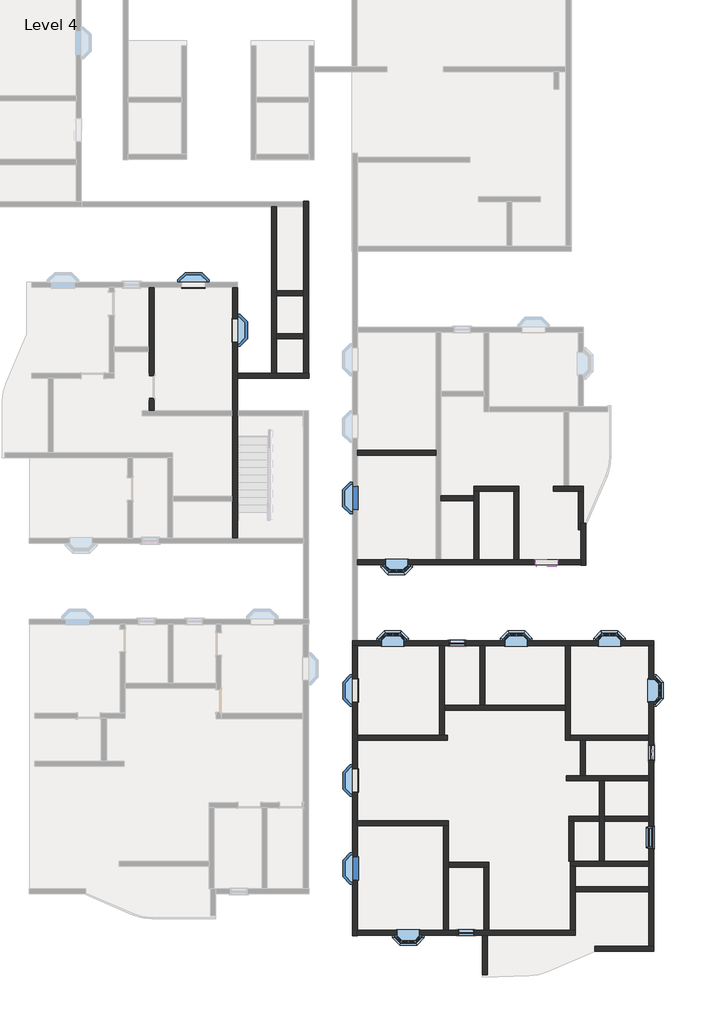
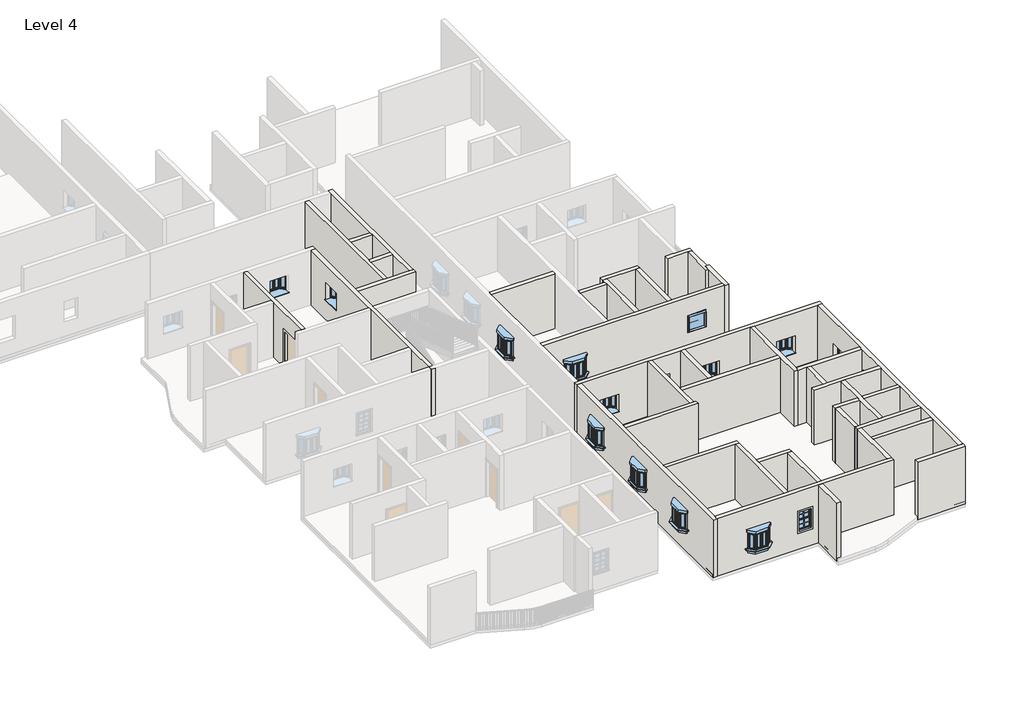
# One storey, part 2 of 14: 40 walls, 17 windows.
"""IFC4 building model written with IfcOpenShell, lengths in millimetres."""

from ifc_helpers import new_model, si_unit, frame, origin, place, context, project, spatial, polyline, outline, extrude, faceted_brep, transform, mapped, element, save
from components import window_910x910mm_67ef725a, window_8debb0fa, windows_sgl_w_glazing_bars_910x910mm_256712d0

model = new_model("IFC4")

# Units and contexts
model_context = context("Model", 3, world=origin())
ifc_project = project(units=[si_unit("LENGTHUNIT", "METRE", prefix="MILLI")], contexts=[model_context])

# Site, building, storey
site = spatial("IfcSite", under=ifc_project)
building = spatial("IfcBuilding", under=site)
storey = spatial("IfcBuildingStorey", under=building, Name="Level 4", Elevation=9144.0)

# Walls
placement = place(None, origin())
element("IfcWall", 1, ObjectType="4.5\" p", at=placement, inside=storey, context=model_context, shape_type="SweptSolid", body=[
    extrude(outline(polyline([(6070.4380523, -28382.7374148), (6070.4380523, -26796.6042694), (6273.6380523, -26796.6042694), (6273.6380523, -28382.7374148), (6070.4380523, -28382.7374148)])), frame((0.0, 0.0, 9144.0), z_axis=(0.0, 0.0, 1.0), x_axis=(1.0, 0.0, 0.0)), (0.0, 0.0, 1.0), 3048.0),
])
element("IfcWall", 2, ObjectType="4.5\" p", at=placement, inside=storey, context=model_context, shape_type="Brep", body=[
    faceted_brep([(10639.6896214, -27431.6042694, 9144.0), (13030.0380523, -27431.6042694, 9144.0), (13030.0380523, -27431.6042694, 12192.0), (10639.6896214, -27431.6042694, 12192.0), (10639.6896214, -27228.4042694, 9144.0), (10639.6896214, -27228.4042694, 12192.0), (12814.1380523, -27228.4042694, 12192.0), (13017.3380523, -27228.4042694, 12192.0), (13030.0380523, -27228.4042694, 12192.0), (13030.0380523, -27228.4042694, 9144.0), (13017.3380523, -27228.4042694, 9144.0), (12814.1380523, -27228.4042694, 9144.0)], [[[0, 1, 2, 3]], [[4, 5, 6, 7, 8, 9, 10, 11]], [[1, 0, 4, 11, 10, 9]], [[2, 1, 9, 8]], [[3, 2, 8, 7, 6, 5]], [[0, 3, 5, 4]]]),
])
element("IfcWall", 3, ObjectType="4.5\" p", at=placement, inside=storey, context=model_context, shape_type="Brep", body=[
    faceted_brep([(1015.8380523, -18878.1542694, 9144.0), (4648.0380523, -18878.1542694, 9144.0), (4648.0380523, -18878.1542694, 12192.0), (1015.8380523, -18878.1542694, 12192.0), (1015.8380523, -18674.9542694, 9144.0), (1015.8380523, -18674.9542694, 12192.0), (4336.8880523, -18674.9542694, 12192.0), (4540.0880523, -18674.9542694, 12192.0), (4648.0380523, -18674.9542694, 12192.0), (4648.0380523, -18674.9542694, 9144.0), (4540.0880523, -18674.9542694, 9144.0), (4336.8880523, -18674.9542694, 9144.0)], [[[0, 1, 2, 3]], [[4, 5, 6, 7, 8, 9, 10, 11]], [[1, 0, 4, 11, 10, 9]], [[2, 1, 9, 8]], [[3, 2, 8, 7, 6, 5]], [[0, 3, 5, 4]]]),
])
element("IfcWall", 4, ObjectType="4.5\" p", at=placement, inside=storey, context=model_context, shape_type="Brep", body=[
    faceted_brep([(4336.8880523, -15049.1042694, 9144.0), (4336.8880523, -18674.9542694, 9144.0), (4336.8880523, -18674.9542694, 12192.0), (4336.8880523, -15049.1042694, 12192.0), (4540.0880523, -15049.1042694, 9144.0), (4540.0880523, -15049.1042694, 12192.0), (4540.0880523, -17455.7542694, 12192.0), (4540.0880523, -17658.9542694, 12192.0), (4540.0880523, -18674.9542694, 12192.0), (4540.0880523, -18674.9542694, 9144.0), (4540.0880523, -17658.9542694, 9144.0), (4540.0880523, -17455.7542694, 9144.0)], [[[0, 1, 2, 3]], [[4, 5, 6, 7, 8, 9, 10, 11]], [[1, 0, 4, 11, 10, 9]], [[3, 2, 8, 7, 6, 5]], [[0, 3, 5, 4]], [[2, 1, 9, 8]]]),
])
element("IfcWall", 5, ObjectType="4.5\" p", at=placement, inside=storey, context=model_context, shape_type="Brep", body=[
    faceted_brep([(4540.0880523, -17658.9542694, 9144.0), (9442.2880523, -17658.9542694, 9144.0), (9442.2880523, -17658.9542694, 12192.0), (4540.0880523, -17658.9542694, 12192.0), (4540.0880523, -17455.7542694, 9144.0), (4540.0880523, -17455.7542694, 12192.0), (5975.1880523, -17455.7542694, 12192.0), (6178.3880523, -17455.7542694, 12192.0), (9442.2880523, -17455.7542694, 12192.0), (9442.2880523, -17455.7542694, 9144.0), (6178.3880523, -17455.7542694, 9144.0), (5975.1880523, -17455.7542694, 9144.0)], [[[0, 1, 2, 3]], [[4, 5, 6, 7, 8, 9, 10, 11]], [[1, 0, 4, 11, 10, 9]], [[3, 2, 8, 7, 6, 5]], [[0, 3, 5, 4]], [[2, 1, 9, 8]]]),
])
element("IfcWall", 6, ObjectType="4.5\" p", at=placement, inside=storey, context=model_context, shape_type="SweptSolid", body=[
    extrude(outline(polyline([(5975.1880523, -17455.7542694), (5975.1880523, -15049.1042694), (6178.3880523, -15049.1042694), (6178.3880523, -17455.7542694), (5975.1880523, -17455.7542694)])), frame((0.0, 0.0, 9144.0), z_axis=(0.0, 0.0, 1.0), x_axis=(1.0, 0.0, 0.0)), (0.0, 0.0, 1.0), 3048.0),
])
element("IfcWall", 7, ObjectType="4.5\" p", at=placement, inside=storey, context=model_context, shape_type="Brep", body=[
    faceted_brep([(9442.2880523, -15049.1042694, 9144.0), (9442.2880523, -17455.7542694, 9144.0), (9442.2880523, -17658.9542694, 9144.0), (9442.2880523, -18871.8042694, 9144.0), (9442.2880523, -18871.8042694, 12192.0), (9442.2880523, -17658.9542694, 12192.0), (9442.2880523, -17455.7542694, 12192.0), (9442.2880523, -15049.1042694, 12192.0), (9645.4880523, -15049.1042694, 9144.0), (9645.4880523, -15049.1042694, 12192.0), (9645.4880523, -18668.6042694, 12192.0), (9645.4880523, -18871.8042694, 12192.0), (9645.4880523, -18871.8042694, 9144.0), (9645.4880523, -18668.6042694, 9144.0)], [[[0, 1, 2, 3, 4, 5, 6, 7]], [[8, 9, 10, 11, 12, 13]], [[3, 2, 1, 0, 8, 13, 12]], [[7, 6, 5, 4, 11, 10, 9]], [[0, 7, 9, 8]], [[4, 3, 12, 11]]]),
])
element("IfcWall", 8, ObjectType="4.5\" p", at=placement, inside=storey, context=model_context, shape_type="Brep", body=[
    faceted_brep([(1015.8380523, -22345.2542694, 9144.0), (4489.2880523, -22345.2542694, 9144.0), (4692.4880523, -22345.2542694, 9144.0), (4692.4880523, -22345.2542694, 12192.0), (4489.2880523, -22345.2542694, 12192.0), (1015.8380523, -22345.2542694, 12192.0), (1015.8380523, -22142.0542694, 9144.0), (1015.8380523, -22142.0542694, 12192.0), (4692.4880523, -22142.0542694, 12192.0), (4692.4880523, -22142.0542694, 9144.0)], [[[0, 1, 2, 3, 4, 5]], [[6, 7, 8, 9]], [[2, 1, 0, 6, 9]], [[5, 4, 3, 8, 7]], [[0, 5, 7, 6]], [[3, 2, 9, 8]]]),
])
element("IfcWall", 9, ObjectType="4.5\" p", at=placement, inside=storey, context=model_context, shape_type="Brep", body=[
    faceted_brep([(4489.2880523, -22345.2542694, 9144.0), (4489.2880523, -26580.7042694, 9144.0), (4489.2880523, -26580.7042694, 12192.0), (4489.2880523, -22345.2542694, 12192.0), (4692.4880523, -22345.2542694, 9144.0), (4692.4880523, -22345.2542694, 12192.0), (4692.4880523, -23818.4542694, 12192.0), (4692.4880523, -24021.6542694, 12192.0), (4692.4880523, -26580.7042694, 12192.0), (4692.4880523, -26580.7042694, 9144.0), (4692.4880523, -24021.6542694, 9144.0), (4692.4880523, -23818.4542694, 9144.0)], [[[0, 1, 2, 3]], [[4, 5, 6, 7, 8, 9, 10, 11]], [[1, 0, 4, 11, 10, 9]], [[3, 2, 8, 7, 6, 5]], [[0, 3, 5, 4]], [[2, 1, 9, 8]]]),
])
element("IfcWall", 10, ObjectType="4.5\" p", at=placement, inside=storey, context=model_context, shape_type="Brep", body=[
    faceted_brep([(4692.4880523, -24021.6542694, 9144.0), (6127.5880523, -24021.6542694, 9144.0), (6330.7880523, -24021.6542694, 9144.0), (6330.7880523, -24021.6542694, 12192.0), (6127.5880523, -24021.6542694, 12192.0), (4692.4880523, -24021.6542694, 12192.0), (4692.4880523, -23818.4542694, 9144.0), (4692.4880523, -23818.4542694, 12192.0), (6330.7880523, -23818.4542694, 12192.0), (6330.7880523, -23818.4542694, 9144.0)], [[[0, 1, 2, 3, 4, 5]], [[6, 7, 8, 9]], [[2, 1, 0, 6, 9]], [[5, 4, 3, 8, 7]], [[0, 5, 7, 6]], [[3, 2, 9, 8]]]),
])
element("IfcWall", 11, ObjectType="4.5\" p", at=placement, inside=storey, context=model_context, shape_type="SweptSolid", body=[
    extrude(outline(polyline([(6127.5880523, -26580.7042694), (6127.5880523, -24021.6542694), (6330.7880523, -24021.6542694), (6330.7880523, -26580.7042694), (6127.5880523, -26580.7042694)])), frame((0.0, 0.0, 9144.0), z_axis=(0.0, 0.0, 1.0), x_axis=(1.0, 0.0, 0.0)), (0.0, 0.0, 1.0), 3048.0),
])
element("IfcWall", 12, ObjectType="4.5\" p", at=placement, inside=storey, context=model_context, shape_type="Brep", body=[
    faceted_brep([(9645.4880523, -18871.8042694, 9144.0), (10051.8880523, -18871.8042694, 9144.0), (10255.0880523, -18871.8042694, 9144.0), (12814.1380523, -18871.8042694, 9144.0), (12814.1380523, -18871.8042694, 12192.0), (10255.0880523, -18871.8042694, 12192.0), (10051.8880523, -18871.8042694, 12192.0), (9645.4880523, -18871.8042694, 12192.0), (9645.4880523, -18668.6042694, 9144.0), (9645.4880523, -18668.6042694, 12192.0), (12814.1380523, -18668.6042694, 12192.0), (12814.1380523, -18668.6042694, 9144.0)], [[[0, 1, 2, 3, 4, 5, 6, 7]], [[8, 9, 10, 11]], [[3, 2, 1, 0, 8, 11]], [[7, 6, 5, 4, 10, 9]], [[0, 7, 9, 8]], [[4, 3, 11, 10]]]),
])
element("IfcWall", 13, ObjectType="4.5\" p", at=placement, inside=storey, context=model_context, shape_type="SweptSolid", body=[
    extrude(outline(polyline([(10051.8880523, -20313.2542694), (10051.8880523, -18871.8042694), (10255.0880523, -18871.8042694), (10255.0880523, -20313.2542694), (10051.8880523, -20313.2542694)])), frame((0.0, 0.0, 9144.0), z_axis=(0.0, 0.0, 1.0), x_axis=(1.0, 0.0, 0.0)), (0.0, 0.0, 1.0), 3048.0),
])
element("IfcWall", 14, ObjectType="4.5\" p", at=placement, inside=storey, context=model_context, shape_type="Brep", body=[
    faceted_brep([(12814.1380523, -20313.2542694, 9144.0), (10255.0880523, -20313.2542694, 9144.0), (10051.8880523, -20313.2542694, 9144.0), (9486.7380523, -20313.2542694, 9144.0), (9486.7380523, -20313.2542694, 12192.0), (10051.8880523, -20313.2542694, 12192.0), (10255.0880523, -20313.2542694, 12192.0), (12814.1380523, -20313.2542694, 12192.0), (12814.1380523, -20516.4542694, 9144.0), (12814.1380523, -20516.4542694, 12192.0), (11017.0880523, -20516.4542694, 12192.0), (10813.8880523, -20516.4542694, 12192.0), (9486.7380523, -20516.4542694, 12192.0), (9486.7380523, -20516.4542694, 9144.0), (10813.8880523, -20516.4542694, 9144.0), (11017.0880523, -20516.4542694, 9144.0)], [[[0, 1, 2, 3, 4, 5, 6, 7]], [[8, 9, 10, 11, 12, 13, 14, 15]], [[3, 2, 1, 0, 8, 15, 14, 13]], [[4, 3, 13, 12]], [[7, 6, 5, 4, 12, 11, 10, 9]], [[0, 7, 9, 8]]]),
])
element("IfcWall", 15, ObjectType="4.5\" p", at=placement, inside=storey, context=model_context, shape_type="Brep", body=[
    faceted_brep([(10813.8880523, -20516.4542694, 9144.0), (10813.8880523, -21951.5542694, 9144.0), (10813.8880523, -22154.7542694, 9144.0), (10813.8880523, -23779.5416506, 9144.0), (10813.8880523, -23779.5416506, 12192.0), (10813.8880523, -22154.7542694, 12192.0), (10813.8880523, -21951.5542694, 12192.0), (10813.8880523, -20516.4542694, 12192.0), (11017.0880523, -20516.4542694, 9144.0), (11017.0880523, -20516.4542694, 12192.0), (11017.0880523, -21951.5542694, 12192.0), (11017.0880523, -22154.7542694, 12192.0), (11017.0880523, -23779.5416506, 12192.0), (11017.0880523, -23779.5416506, 9144.0), (11017.0880523, -22154.7542694, 9144.0), (11017.0880523, -21951.5542694, 9144.0)], [[[0, 1, 2, 3, 4, 5, 6, 7]], [[8, 9, 10, 11, 12, 13, 14, 15]], [[3, 2, 1, 0, 8, 15, 14, 13]], [[7, 6, 5, 4, 12, 11, 10, 9]], [[0, 7, 9, 8]], [[4, 3, 13, 12]]]),
])
element("IfcWall", 16, ObjectType="4.5\" p", at=placement, inside=storey, context=model_context, shape_type="Brep", body=[
    faceted_brep([(12814.1380523, -23779.5416506, 9144.0), (11017.0880523, -23779.5416506, 9144.0), (10813.8880523, -23779.5416506, 9144.0), (9791.5380523, -23779.5416506, 9144.0), (9632.7880523, -23779.5416506, 9144.0), (9632.7880523, -23779.5416506, 12192.0), (9791.5380523, -23779.5416506, 12192.0), (10813.8880523, -23779.5416506, 12192.0), (11017.0880523, -23779.5416506, 12192.0), (12814.1380523, -23779.5416506, 12192.0), (12814.1380523, -23982.7416506, 9144.0), (12814.1380523, -23982.7416506, 12192.0), (9835.9880523, -23982.7416506, 12192.0), (9632.7880523, -23982.7416506, 12192.0), (9632.7880523, -23982.7416506, 9144.0), (9835.9880523, -23982.7416506, 9144.0)], [[[0, 1, 2, 3, 4, 5, 6, 7, 8, 9]], [[10, 11, 12, 13, 14, 15]], [[4, 3, 2, 1, 0, 10, 15, 14]], [[9, 8, 7, 6, 5, 13, 12, 11]], [[0, 9, 11, 10]], [[5, 4, 14, 13]]]),
])
element("IfcWall", 17, ObjectType="4.5\" p", at=placement, inside=storey, context=model_context, shape_type="Brep", body=[
    faceted_brep([(9632.7880523, -23982.7416506, 9144.0), (9632.7880523, -26580.7042694, 9144.0), (9632.7880523, -26580.7042694, 12192.0), (9632.7880523, -23982.7416506, 12192.0), (9835.9880523, -23982.7416506, 9144.0), (9835.9880523, -23982.7416506, 12192.0), (9835.9880523, -24805.3496998, 12192.0), (9835.9880523, -25008.5496998, 12192.0), (9835.9880523, -26580.7042694, 12192.0), (9835.9880523, -26580.7042694, 9144.0), (9835.9880523, -25008.5496998, 9144.0), (9835.9880523, -24805.3496998, 9144.0)], [[[0, 1, 2, 3]], [[4, 5, 6, 7, 8, 9, 10, 11]], [[1, 0, 4, 11, 10, 9]], [[3, 2, 8, 7, 6, 5]], [[2, 1, 9, 8]], [[0, 3, 5, 4]]]),
])
element("IfcWall", 18, ObjectType="4.5\" p", at=placement, inside=storey, context=model_context, shape_type="SweptSolid", body=[
    extrude(outline(polyline([(12814.1380523, -25008.5496998), (9835.9880523, -25008.5496998), (9835.9880523, -24805.3496998), (12814.1380523, -24805.3496998), (12814.1380523, -25008.5496998)])), frame((0.0, 0.0, 9144.0), z_axis=(0.0, 0.0, 1.0), x_axis=(1.0, 0.0, 0.0)), (0.0, 0.0, 1.0), 3048.0),
])
element("IfcWall", 19, ObjectType="4.5\" p", at=placement, inside=storey, context=model_context, shape_type="Brep", body=[
    faceted_brep([(-7432.737215, -5015.2916506, 11277.6), (-7432.737215, -5015.2916506, 9144.0), (-7432.737215, -5523.2916506, 9144.0), (-7432.737215, -5523.2916506, 12192.0), (-7432.737215, -3135.6916506, 12192.0), (-7432.737215, -2932.4916506, 12192.0), (-7432.737215, -525.8416506, 12192.0), (-7432.737215, -525.8416506, 9144.0), (-7432.737215, -2932.4916506, 9144.0), (-7432.737215, -3135.6916506, 9144.0), (-7432.737215, -4100.8916506, 9144.0), (-7432.737215, -4100.8916506, 11277.6), (-7229.537215, -5523.2916506, 9144.0), (-7229.537215, -5015.2916506, 9144.0), (-7229.537215, -5015.2916506, 11277.6), (-7229.537215, -4100.8916506, 11277.6), (-7229.537215, -4100.8916506, 9144.0), (-7229.537215, -525.8416506, 9144.0), (-7229.537215, -525.8416506, 12192.0), (-7229.537215, -5523.2916506, 12192.0)], [[[0, 1, 2, 3, 4, 5, 6, 7, 8, 9, 10, 11]], [[12, 13, 14, 15, 16, 17, 18, 19]], [[2, 1, 13, 12]], [[10, 9, 8, 7, 17, 16]], [[6, 5, 4, 3, 19, 18]], [[7, 6, 18, 17]], [[3, 2, 12, 19]], [[14, 13, 1, 0]], [[15, 14, 0, 11]], [[16, 15, 11, 10]]]),
])
element("IfcWall", 20, ObjectType="4.5\" p", at=placement, inside=storey, context=model_context, shape_type="Brep", body=[
    faceted_brep([(-3857.687215, -4202.4916506, 9144.0), (-961.4891351, -4202.4916506, 9144.0), (-961.4891351, -4202.4916506, 12192.0), (-3857.687215, -4202.4916506, 12192.0), (-3857.687215, -3999.2916506, 9144.0), (-3857.687215, -3999.2916506, 12192.0), (-2472.7891351, -3999.2916506, 12192.0), (-2269.5891351, -3999.2916506, 12192.0), (-1177.3891351, -3999.2916506, 12192.0), (-974.1891351, -3999.2916506, 12192.0), (-961.4891351, -3999.2916506, 12192.0), (-961.4891351, -3999.2916506, 9144.0), (-974.1891351, -3999.2916506, 9144.0), (-1177.3891351, -3999.2916506, 9144.0), (-2269.5891351, -3999.2916506, 9144.0), (-2472.7891351, -3999.2916506, 9144.0)], [[[0, 1, 2, 3]], [[4, 5, 6, 7, 8, 9, 10, 11, 12, 13, 14, 15]], [[1, 0, 4, 15, 14, 13, 12, 11]], [[2, 1, 11, 10]], [[3, 2, 10, 9, 8, 7, 6, 5]], [[0, 3, 5, 4]]]),
])
element("IfcWall", 21, ObjectType="4.5\" p", at=placement, inside=storey, context=model_context, shape_type="SweptSolid", body=[
    extrude(outline(polyline([(-1177.3891351, -868.7416506), (-2269.5891351, -868.7416506), (-2269.5891351, -665.5416506), (-1177.3891351, -665.5416506), (-1177.3891351, -868.7416506)])), frame((0.0, 0.0, 9144.0), z_axis=(0.0, 0.0, 1.0), x_axis=(1.0, 0.0, 0.0)), (0.0, 0.0, 1.0), 3048.0),
])
element("IfcWall", 22, ObjectType="4.5\" p", at=placement, inside=storey, context=model_context, shape_type="SweptSolid", body=[
    extrude(outline(polyline([(-1177.3891351, -2597.8466506), (-2269.5891351, -2597.8466506), (-2269.5891351, -2394.6466506), (-1177.3891351, -2394.6466506), (-1177.3891351, -2597.8466506)])), frame((0.0, 0.0, 9144.0), z_axis=(0.0, 0.0, 1.0), x_axis=(1.0, 0.0, 0.0)), (0.0, 0.0, 1.0), 3048.0),
])
element("IfcWall", 23, ObjectType="4.5\" p", at=placement, inside=storey, context=model_context, shape_type="SweptSolid", body=[
    extrude(outline(polyline([(5721.1880523, -9162.6542694), (4387.6880523, -9162.6542694), (4387.6880523, -8959.4542694), (5721.1880523, -8959.4542694), (5721.1880523, -9162.6542694)])), frame((0.0, 0.0, 9144.0), z_axis=(0.0, 0.0, 1.0), x_axis=(1.0, 0.0, 0.0)), (0.0, 0.0, 1.0), 3048.0),
])
element("IfcWall", 24, ObjectType="4.5\" p", at=placement, inside=storey, context=model_context, shape_type="Brep", body=[
    faceted_brep([(5721.1880523, -8781.6542694, 9144.0), (5924.3880523, -8781.6542694, 9144.0), (7359.4880523, -8781.6542694, 9144.0), (7562.6880523, -8781.6542694, 9144.0), (7562.6880523, -8781.6542694, 12192.0), (7359.4880523, -8781.6542694, 12192.0), (5924.3880523, -8781.6542694, 12192.0), (5721.1880523, -8781.6542694, 12192.0), (5721.1880523, -8578.4542694, 9144.0), (5721.1880523, -8578.4542694, 12192.0), (7562.6880523, -8578.4542694, 12192.0), (7562.6880523, -8578.4542694, 9144.0)], [[[0, 1, 2, 3, 4, 5, 6, 7]], [[8, 9, 10, 11]], [[3, 2, 1, 0, 8, 11]], [[7, 6, 5, 4, 10, 9]], [[0, 7, 9, 8]], [[4, 3, 11, 10]]]),
])
element("IfcWall", 25, ObjectType="4.5\" p", at=placement, inside=storey, context=model_context, shape_type="Brep", body=[
    faceted_brep([(5721.1880523, -8781.6542694, 9144.0), (5721.1880523, -8959.4542694, 9144.0), (5721.1880523, -9162.6542694, 9144.0), (5721.1880523, -11556.6042694, 9144.0), (5721.1880523, -11556.6042694, 12192.0), (5721.1880523, -9162.6542694, 12192.0), (5721.1880523, -8959.4542694, 12192.0), (5721.1880523, -8781.6542694, 12192.0), (5924.3880523, -8781.6542694, 9144.0), (5924.3880523, -8781.6542694, 12192.0), (5924.3880523, -11556.6042694, 12192.0), (5924.3880523, -11556.6042694, 9144.0)], [[[0, 1, 2, 3, 4, 5, 6, 7]], [[8, 9, 10, 11]], [[3, 2, 1, 0, 8, 11]], [[7, 6, 5, 4, 10, 9]], [[0, 7, 9, 8]], [[4, 3, 11, 10]]]),
])
element("IfcWall", 26, ObjectType="4.5\" p", at=placement, inside=storey, context=model_context, shape_type="SweptSolid", body=[
    extrude(outline(polyline([(7359.4880523, -11556.6042694), (7359.4880523, -8781.6542694), (7562.6880523, -8781.6542694), (7562.6880523, -11556.6042694), (7359.4880523, -11556.6042694)])), frame((0.0, 0.0, 9144.0), z_axis=(0.0, 0.0, 1.0), x_axis=(1.0, 0.0, 0.0)), (0.0, 0.0, 1.0), 3048.0),
])
element("IfcWall", 27, ObjectType="4.5\" p", at=placement, inside=storey, context=model_context, shape_type="SweptSolid", body=[
    extrude(outline(polyline([(4184.4880523, -7333.8542694), (1007.0108649, -7333.8542694), (1007.0108649, -7130.6542694), (4184.4880523, -7130.6542694), (4184.4880523, -7333.8542694)])), frame((0.0, 0.0, 9144.0), z_axis=(0.0, 0.0, 1.0), x_axis=(1.0, 0.0, 0.0)), (0.0, 0.0, 1.0), 3048.0),
])
element("IfcWall", 28, ObjectType="4.5\" p", at=placement, inside=storey, context=model_context, shape_type="Brep", body=[
    faceted_brep([(8953.3380523, -8781.6542694, 9144.0), (9956.6380523, -8781.6542694, 9144.0), (10159.8380523, -8781.6542694, 9144.0), (10172.5380523, -8781.6542694, 9144.0), (10172.5380523, -8781.6542694, 12192.0), (10159.8380523, -8781.6542694, 12192.0), (9956.6380523, -8781.6542694, 12192.0), (8953.3380523, -8781.6542694, 12192.0), (8953.3380523, -8578.4542694, 9144.0), (8953.3380523, -8578.4542694, 12192.0), (9371.2322031, -8578.4542694, 12192.0), (9574.4322031, -8578.4542694, 12192.0), (10172.5380523, -8578.4542694, 12192.0), (10172.5380523, -8578.4542694, 9144.0), (9574.4322031, -8578.4542694, 9144.0), (9371.2322031, -8578.4542694, 9144.0)], [[[0, 1, 2, 3, 4, 5, 6, 7]], [[8, 9, 10, 11, 12, 13, 14, 15]], [[3, 2, 1, 0, 8, 15, 14, 13]], [[4, 3, 13, 12]], [[7, 6, 5, 4, 12, 11, 10, 9]], [[0, 7, 9, 8]]]),
])
element("IfcWall", 29, ObjectType="4.5\" p", at=placement, inside=storey, context=model_context, shape_type="SweptSolid", body=[
    extrude(outline(polyline([(9956.6380523, -10352.8912671), (9956.6380523, -8781.6542694), (10159.8380523, -8781.6542694), (10159.8380523, -10352.8912671), (9956.6380523, -10352.8912671)])), frame((0.0, 0.0, 9144.0), z_axis=(0.0, 0.0, 1.0), x_axis=(1.0, 0.0, 0.0)), (0.0, 0.0, 1.0), 3048.0),
])
element("IfcWall", 30, ObjectType="4.5\" p", at=placement, inside=storey, context=model_context, shape_type="Brep", body=[
    faceted_brep([(12814.1380523, -21951.5542694, 12192.0), (12814.1380523, -21951.5542694, 9144.0), (11017.0880523, -21951.5542694, 9144.0), (11017.0880523, -21951.5542694, 12192.0), (12814.1380523, -22154.7542694, 9144.0), (12814.1380523, -22154.7542694, 12192.0), (11017.0880523, -22154.7542694, 12192.0), (11017.0880523, -22154.7542694, 9144.0)], [[[0, 1, 2, 3]], [[4, 5, 6, 7]], [[1, 4, 7, 2]], [[5, 0, 3, 6]], [[1, 0, 5, 4]], [[3, 2, 7, 6]]]),
    faceted_brep([(9588.3380523, -21951.5542694, 9144.0), (9588.3380523, -21951.5542694, 12192.0), (10813.8880523, -21951.5542694, 12192.0), (10813.8880523, -21951.5542694, 9144.0), (9588.3380523, -22154.7542694, 12192.0), (9588.3380523, -22154.7542694, 9144.0), (9791.5380523, -22154.7542694, 9144.0), (10813.8880523, -22154.7542694, 9144.0), (10813.8880523, -22154.7542694, 12192.0), (9791.5380523, -22154.7542694, 12192.0)], [[[0, 1, 2, 3]], [[4, 5, 6, 7, 8, 9]], [[5, 0, 3, 7, 6]], [[1, 4, 9, 8, 2]], [[3, 2, 8, 7]], [[1, 0, 5, 4]]]),
])
element("IfcWall", 31, ObjectType="4.5\" p", at=placement, inside=storey, context=model_context, shape_type="Brep", body=[
    faceted_brep([(9588.3380523, -22154.7542694, 9144.0), (9588.3380523, -23779.5416506, 9144.0), (9588.3380523, -23779.5416506, 12192.0), (9588.3380523, -22154.7542694, 12192.0), (9791.5380523, -22154.7542694, 9144.0), (9791.5380523, -22154.7542694, 12192.0), (9791.5380523, -23779.5416506, 12192.0), (9791.5380523, -23779.5416506, 9144.0), (9632.7880523, -23779.5416506, 9144.0), (9632.7880523, -23779.5416506, 12192.0)], [[[0, 1, 2, 3]], [[4, 5, 6, 7]], [[1, 0, 4, 7, 8]], [[3, 2, 9, 6, 5]], [[2, 1, 8, 7, 6, 9]], [[0, 3, 5, 4]]]),
])
element("IfcWall", 32, ObjectType="9\"", at=placement, inside=storey, context=model_context, shape_type="Brep", body=[
    faceted_brep([(799.9380523, -15049.1042694, 9144.0), (812.6380523, -15049.1042694, 9144.0), (1015.8380523, -15049.1042694, 9144.0), (4336.8880523, -15049.1042694, 9144.0), (4540.0880523, -15049.1042694, 9144.0), (5975.1880523, -15049.1042694, 9144.0), (6178.3880523, -15049.1042694, 9144.0), (9442.2880523, -15049.1042694, 9144.0), (9645.4880523, -15049.1042694, 9144.0), (12814.1380523, -15049.1042694, 9144.0), (13017.3380523, -15049.1042694, 9144.0), (13030.0380523, -15049.1042694, 9144.0), (13030.0380523, -15049.1042694, 12192.0), (13017.3380523, -15049.1042694, 12192.0), (12814.1380523, -15049.1042694, 12192.0), (9645.4880523, -15049.1042694, 12192.0), (9442.2880523, -15049.1042694, 12192.0), (6178.3880523, -15049.1042694, 12192.0), (5975.1880523, -15049.1042694, 12192.0), (4540.0880523, -15049.1042694, 12192.0), (4336.8880523, -15049.1042694, 12192.0), (1015.8380523, -15049.1042694, 12192.0), (812.6380523, -15049.1042694, 12192.0), (799.9380523, -15049.1042694, 12192.0), (1983.2380523, -15049.1042694, 10968.4), (2893.2380523, -15049.1042694, 10968.4), (2893.2380523, -15049.1042694, 10058.4), (1983.2380523, -15049.1042694, 10058.4), (10774.8130523, -15049.1042694, 10968.4), (11684.8130523, -15049.1042694, 10968.4), (11684.8130523, -15049.1042694, 10058.4), (10774.8130523, -15049.1042694, 10058.4), (6993.3880523, -15049.1042694, 10968.4), (7903.3880523, -15049.1042694, 10968.4), (7903.3880523, -15049.1042694, 10058.4), (6993.3880523, -15049.1042694, 10058.4), (4717.8880523, -15049.1042694, 11125.2), (5378.2880523, -15049.1042694, 11125.2), (5378.2880523, -15049.1042694, 10058.4), (4717.8880523, -15049.1042694, 10058.4), (799.9380523, -14845.9042694, 9144.0), (799.9380523, -14845.9042694, 12192.0), (803.8108649, -14845.9042694, 12192.0), (1007.0108649, -14845.9042694, 12192.0), (13030.0380523, -14845.9042694, 12192.0), (13030.0380523, -14845.9042694, 9144.0), (1007.0108649, -14845.9042694, 9144.0), (803.8108649, -14845.9042694, 9144.0), (1983.2380523, -14845.9042694, 10968.4), (1983.2380523, -14845.9042694, 10058.4), (2893.2380523, -14845.9042694, 10058.4), (2893.2380523, -14845.9042694, 10968.4), (10774.8130523, -14845.9042694, 10968.4), (10774.8130523, -14845.9042694, 10058.4), (11684.8130523, -14845.9042694, 10058.4), (11684.8130523, -14845.9042694, 10968.4), (6993.3880523, -14845.9042694, 10968.4), (6993.3880523, -14845.9042694, 10058.4), (7903.3880523, -14845.9042694, 10058.4), (7903.3880523, -14845.9042694, 10968.4), (4717.8880523, -14845.9042694, 11125.2), (4717.8880523, -14845.9042694, 10058.4), (5378.2880523, -14845.9042694, 10058.4), (5378.2880523, -14845.9042694, 11125.2)], [[[0, 1, 2, 3, 4, 5, 6, 7, 8, 9, 10, 11, 12, 13, 14, 15, 16, 17, 18, 19, 20, 21, 22, 23], [24, 25, 26, 27], [28, 29, 30, 31], [32, 33, 34, 35], [36, 37, 38, 39]], [[40, 41, 42, 43, 44, 45, 46, 47], [48, 49, 50, 51], [52, 53, 54, 55], [56, 57, 58, 59], [60, 61, 62, 63]], [[11, 10, 9, 8, 7, 6, 5, 4, 3, 2, 1, 0, 40, 47, 46, 45]], [[12, 11, 45, 44]], [[23, 22, 21, 20, 19, 18, 17, 16, 15, 14, 13, 12, 44, 43, 42, 41]], [[0, 23, 41, 40]], [[49, 48, 24, 27]], [[50, 49, 27, 26]], [[51, 50, 26, 25]], [[48, 51, 25, 24]], [[53, 52, 28, 31]], [[54, 53, 31, 30]], [[55, 54, 30, 29]], [[52, 55, 29, 28]], [[57, 56, 32, 35]], [[58, 57, 35, 34]], [[59, 58, 34, 33]], [[56, 59, 33, 32]], [[61, 60, 36, 39]], [[62, 61, 39, 38]], [[63, 62, 38, 37]], [[60, 63, 37, 36]]]),
])
element("IfcWall", 33, ObjectType="9\"", at=placement, inside=storey, context=model_context, shape_type="Brep", body=[
    faceted_brep([(12814.1380523, -15049.1042694, 9144.0), (12814.1380523, -18668.6042694, 9144.0), (12814.1380523, -18871.8042694, 9144.0), (12814.1380523, -20313.2542694, 9144.0), (12814.1380523, -20516.4542694, 9144.0), (12814.1380523, -21951.5542694, 9144.0), (12814.1380523, -22154.7542694, 9144.0), (12814.1380523, -23779.5416506, 9144.0), (12814.1380523, -23982.7416506, 9144.0), (12814.1380523, -24805.3496998, 9144.0), (12814.1380523, -25008.5496998, 9144.0), (12814.1380523, -27228.4042694, 9144.0), (12814.1380523, -27228.4042694, 12192.0), (12814.1380523, -25008.5496998, 12192.0), (12814.1380523, -24805.3496998, 12192.0), (12814.1380523, -23982.7416506, 12192.0), (12814.1380523, -23779.5416506, 12192.0), (12814.1380523, -22154.7542694, 12192.0), (12814.1380523, -21951.5542694, 12192.0), (12814.1380523, -20516.4542694, 12192.0), (12814.1380523, -20313.2542694, 12192.0), (12814.1380523, -18871.8042694, 12192.0), (12814.1380523, -18668.6042694, 12192.0), (12814.1380523, -15049.1042694, 12192.0), (12814.1380523, -16403.8542694, 10968.4), (12814.1380523, -17313.8542694, 10968.4), (12814.1380523, -17313.8542694, 10058.4), (12814.1380523, -16403.8542694, 10058.4), (12814.1380523, -23270.1542694, 10968.4), (12814.1380523, -23270.1542694, 10058.4), (12814.1380523, -22360.1542694, 10058.4), (12814.1380523, -22360.1542694, 10968.4), (12814.1380523, -19049.6042694, 11125.2), (12814.1380523, -19710.0042694, 11125.2), (12814.1380523, -19710.0042694, 10058.4), (12814.1380523, -19049.6042694, 10058.4), (13017.3380523, -15049.1042694, 9144.0), (13017.3380523, -15049.1042694, 12192.0), (13017.3380523, -27228.4042694, 12192.0), (13017.3380523, -27228.4042694, 9144.0), (13017.3380523, -16403.8542694, 10968.4), (13017.3380523, -16403.8542694, 10058.4), (13017.3380523, -17313.8542694, 10058.4), (13017.3380523, -17313.8542694, 10968.4), (13017.3380523, -23270.1542694, 10968.4), (13017.3380523, -22360.1542694, 10968.4), (13017.3380523, -22360.1542694, 10058.4), (13017.3380523, -23270.1542694, 10058.4), (13017.3380523, -19049.6042694, 11125.2), (13017.3380523, -19049.6042694, 10058.4), (13017.3380523, -19710.0042694, 10058.4), (13017.3380523, -19710.0042694, 11125.2)], [[[0, 1, 2, 3, 4, 5, 6, 7, 8, 9, 10, 11, 12, 13, 14, 15, 16, 17, 18, 19, 20, 21, 22, 23], [24, 25, 26, 27], [28, 29, 30, 31], [32, 33, 34, 35]], [[36, 37, 38, 39], [40, 41, 42, 43], [44, 45, 46, 47], [48, 49, 50, 51]], [[11, 10, 9, 8, 7, 6, 5, 4, 3, 2, 1, 0, 36, 39]], [[23, 22, 21, 20, 19, 18, 17, 16, 15, 14, 13, 12, 38, 37]], [[0, 23, 37, 36]], [[12, 11, 39, 38]], [[41, 40, 24, 27]], [[42, 41, 27, 26]], [[43, 42, 26, 25]], [[40, 43, 25, 24]], [[29, 28, 44, 47]], [[30, 29, 47, 46]], [[31, 30, 46, 45]], [[28, 31, 45, 44]], [[49, 48, 32, 35]], [[50, 49, 35, 34]], [[51, 50, 34, 33]], [[48, 51, 33, 32]]]),
])
element("IfcWall", 34, ObjectType="9\"", at=placement, inside=storey, context=model_context, shape_type="Brep", body=[
    faceted_brep([(812.6380523, -15049.1042694, 9144.0), (812.6380523, -26796.6042694, 9144.0), (812.6380523, -26796.6042694, 12192.0), (812.6380523, -15049.1042694, 12192.0), (812.6380523, -24527.4542694, 11254.0), (812.6380523, -24527.4542694, 10344.0), (812.6380523, -23617.4542694, 10344.0), (812.6380523, -23617.4542694, 11254.0), (812.6380523, -20965.1042694, 11254.0), (812.6380523, -20965.1042694, 10344.0), (812.6380523, -20055.1042694, 10344.0), (812.6380523, -20055.1042694, 11254.0), (812.6380523, -17317.0292694, 11254.0), (812.6380523, -17317.0292694, 10344.0), (812.6380523, -16407.0292694, 10344.0), (812.6380523, -16407.0292694, 11254.0), (1015.8380523, -15049.1042694, 9144.0), (1015.8380523, -15049.1042694, 12192.0), (1015.8380523, -18674.9542694, 12192.0), (1015.8380523, -18878.1542694, 12192.0), (1015.8380523, -22142.0542694, 12192.0), (1015.8380523, -22345.2542694, 12192.0), (1015.8380523, -26580.7042694, 12192.0), (1015.8380523, -26783.9042694, 12192.0), (1015.8380523, -26796.6042694, 12192.0), (1015.8380523, -26796.6042694, 9144.0), (1015.8380523, -26783.9042694, 9144.0), (1015.8380523, -26580.7042694, 9144.0), (1015.8380523, -22345.2542694, 9144.0), (1015.8380523, -22142.0542694, 9144.0), (1015.8380523, -18878.1542694, 9144.0), (1015.8380523, -18674.9542694, 9144.0), (1015.8380523, -24527.4542694, 11254.0), (1015.8380523, -23617.4542694, 11254.0), (1015.8380523, -23617.4542694, 10344.0), (1015.8380523, -24527.4542694, 10344.0), (1015.8380523, -20965.1042694, 11254.0), (1015.8380523, -20055.1042694, 11254.0), (1015.8380523, -20055.1042694, 10344.0), (1015.8380523, -20965.1042694, 10344.0), (1015.8380523, -17317.0292694, 11254.0), (1015.8380523, -16407.0292694, 11254.0), (1015.8380523, -16407.0292694, 10344.0), (1015.8380523, -17317.0292694, 10344.0)], [[[0, 1, 2, 3], [4, 5, 6, 7], [8, 9, 10, 11], [12, 13, 14, 15]], [[16, 17, 18, 19, 20, 21, 22, 23, 24, 25, 26, 27, 28, 29, 30, 31], [32, 33, 34, 35], [36, 37, 38, 39], [40, 41, 42, 43]], [[1, 0, 16, 31, 30, 29, 28, 27, 26, 25]], [[2, 1, 25, 24]], [[3, 2, 24, 23, 22, 21, 20, 19, 18, 17]], [[0, 3, 17, 16]], [[5, 4, 32, 35]], [[6, 5, 35, 34]], [[7, 6, 34, 33]], [[4, 7, 33, 32]], [[9, 8, 36, 39]], [[10, 9, 39, 38]], [[11, 10, 38, 37]], [[8, 11, 37, 36]], [[13, 12, 40, 43]], [[14, 13, 43, 42]], [[15, 14, 42, 41]], [[12, 15, 41, 40]]]),
])
element("IfcWall", 35, ObjectType="9\"", at=placement, inside=storey, context=model_context, shape_type="Brep", body=[
    faceted_brep([(1015.8380523, -26783.9042694, 9144.0), (9835.9880523, -26783.9042694, 9144.0), (9835.9880523, -26783.9042694, 12192.0), (1015.8380523, -26783.9042694, 12192.0), (3521.8880523, -26783.9042694, 10968.4), (3521.8880523, -26783.9042694, 10058.4), (2611.8880523, -26783.9042694, 10058.4), (2611.8880523, -26783.9042694, 10968.4), (5079.8380523, -26783.9042694, 11125.2), (5740.2380523, -26783.9042694, 11125.2), (5740.2380523, -26783.9042694, 10058.4), (5079.8380523, -26783.9042694, 10058.4), (1015.8380523, -26580.7042694, 9144.0), (1015.8380523, -26580.7042694, 12192.0), (4489.2880523, -26580.7042694, 12192.0), (4692.4880523, -26580.7042694, 12192.0), (6127.5880523, -26580.7042694, 12192.0), (6330.7880523, -26580.7042694, 12192.0), (9632.7880523, -26580.7042694, 12192.0), (9835.9880523, -26580.7042694, 12192.0), (9835.9880523, -26580.7042694, 9144.0), (9632.7880523, -26580.7042694, 9144.0), (6330.7880523, -26580.7042694, 9144.0), (6127.5880523, -26580.7042694, 9144.0), (4692.4880523, -26580.7042694, 9144.0), (4489.2880523, -26580.7042694, 9144.0), (3521.8880523, -26580.7042694, 10968.4), (2611.8880523, -26580.7042694, 10968.4), (2611.8880523, -26580.7042694, 10058.4), (3521.8880523, -26580.7042694, 10058.4), (5079.8380523, -26580.7042694, 11125.2), (5079.8380523, -26580.7042694, 10058.4), (5740.2380523, -26580.7042694, 10058.4), (5740.2380523, -26580.7042694, 11125.2)], [[[0, 1, 2, 3], [4, 5, 6, 7], [8, 9, 10, 11]], [[12, 13, 14, 15, 16, 17, 18, 19, 20, 21, 22, 23, 24, 25], [26, 27, 28, 29], [30, 31, 32, 33]], [[1, 0, 12, 25, 24, 23, 22, 21, 20]], [[3, 2, 19, 18, 17, 16, 15, 14, 13]], [[0, 3, 13, 12]], [[2, 1, 20, 19]], [[5, 4, 26, 29]], [[6, 5, 29, 28]], [[7, 6, 28, 27]], [[4, 7, 27, 26]], [[31, 30, 8, 11]], [[32, 31, 11, 10]], [[33, 32, 10, 9]], [[30, 33, 9, 8]]]),
])
element("IfcWall", 36, ObjectType="9\" w", at=placement, inside=storey, context=model_context, shape_type="Brep", body=[
    faceted_brep([(-4060.887215, -525.8416506, 9144.0), (-4060.887215, -5523.2916506, 9144.0), (-4060.887215, -5726.4916506, 9144.0), (-4060.887215, -8990.3916506, 9144.0), (-4060.887215, -9193.5916506, 9144.0), (-4060.887215, -10901.7416506, 9144.0), (-4060.887215, -10901.7416506, 12192.0), (-4060.887215, -9193.5916506, 12192.0), (-4060.887215, -8990.3916506, 12192.0), (-4060.887215, -5726.4916506, 12192.0), (-4060.887215, -5523.2916506, 12192.0), (-4060.887215, -525.8416506, 12192.0), (-4060.887215, -1807.5666506, 11254.0), (-4060.887215, -2717.5666506, 11254.0), (-4060.887215, -2717.5666506, 10344.0), (-4060.887215, -1807.5666506, 10344.0), (-3857.687215, -525.8416506, 9144.0), (-3857.687215, -525.8416506, 12192.0), (-3857.687215, -3999.2916506, 12192.0), (-3857.687215, -4202.4916506, 12192.0), (-3857.687215, -5523.2916506, 12192.0), (-3857.687215, -5726.4916506, 12192.0), (-3857.687215, -10901.7416506, 12192.0), (-3857.687215, -10901.7416506, 9144.0), (-3857.687215, -5726.4916506, 9144.0), (-3857.687215, -5523.2916506, 9144.0), (-3857.687215, -4202.4916506, 9144.0), (-3857.687215, -3999.2916506, 9144.0), (-3857.687215, -1807.5666506, 11254.0), (-3857.687215, -1807.5666506, 10344.0), (-3857.687215, -2717.5666506, 10344.0), (-3857.687215, -2717.5666506, 11254.0)], [[[0, 1, 2, 3, 4, 5, 6, 7, 8, 9, 10, 11], [12, 13, 14, 15]], [[16, 17, 18, 19, 20, 21, 22, 23, 24, 25, 26, 27], [28, 29, 30, 31]], [[5, 4, 3, 2, 1, 0, 16, 27, 26, 25, 24, 23]], [[6, 5, 23, 22]], [[11, 10, 9, 8, 7, 6, 22, 21, 20, 19, 18, 17]], [[0, 11, 17, 16]], [[29, 28, 12, 15]], [[30, 29, 15, 14]], [[31, 30, 14, 13]], [[28, 31, 13, 12]]]),
])
element("IfcWall", 37, ObjectType="9\" w", at=placement, inside=storey, context=model_context, shape_type="Brep", body=[
    faceted_brep([(-2269.5891351, -3999.2916506, 9144.0), (-2269.5891351, -2597.8466506, 9144.0), (-2269.5891351, -2394.6466506, 9144.0), (-2269.5891351, -868.7416506, 9144.0), (-2269.5891351, -665.5416506, 9144.0), (-2269.5891351, 2750.7583494, 9144.0), (-2269.5891351, 2750.7583494, 12192.0), (-2269.5891351, -665.5416506, 12192.0), (-2269.5891351, -868.7416506, 12192.0), (-2269.5891351, -2394.6466506, 12192.0), (-2269.5891351, -2597.8466506, 12192.0), (-2269.5891351, -3999.2916506, 12192.0), (-2472.7891351, -3999.2916506, 9144.0), (-2472.7891351, -3999.2916506, 12192.0), (-2472.7891351, 2750.7583494, 12192.0), (-2472.7891351, 2750.7583494, 9144.0)], [[[0, 1, 2, 3, 4, 5, 6, 7, 8, 9, 10, 11]], [[12, 13, 14, 15]], [[5, 4, 3, 2, 1, 0, 12, 15]], [[11, 10, 9, 8, 7, 6, 14, 13]], [[0, 11, 13, 12]], [[6, 5, 15, 14]]]),
])
element("IfcWall", 38, ObjectType="9\" w", at=placement, inside=storey, context=model_context, shape_type="Brep", body=[
    faceted_brep([(-974.1891351, -3999.2916506, 9144.0), (-974.1891351, 2966.6583494, 9144.0), (-974.1891351, 2966.6583494, 12192.0), (-974.1891351, -3999.2916506, 12192.0), (-1177.3891351, -3999.2916506, 9144.0), (-1177.3891351, -3999.2916506, 12192.0), (-1177.3891351, -2597.8466506, 12192.0), (-1177.3891351, -2394.6466506, 12192.0), (-1177.3891351, -868.7416506, 12192.0), (-1177.3891351, -665.5416506, 12192.0), (-1177.3891351, 2750.7583494, 12192.0), (-1177.3891351, 2953.9583494, 12192.0), (-1177.3891351, 2966.6583494, 12192.0), (-1177.3891351, 2966.6583494, 9144.0), (-1177.3891351, 2953.9583494, 9144.0), (-1177.3891351, 2750.7583494, 9144.0), (-1177.3891351, -665.5416506, 9144.0), (-1177.3891351, -868.7416506, 9144.0), (-1177.3891351, -2394.6466506, 9144.0), (-1177.3891351, -2597.8466506, 9144.0)], [[[0, 1, 2, 3]], [[4, 5, 6, 7, 8, 9, 10, 11, 12, 13, 14, 15, 16, 17, 18, 19]], [[1, 0, 4, 19, 18, 17, 16, 15, 14, 13]], [[2, 1, 13, 12]], [[3, 2, 12, 11, 10, 9, 8, 7, 6, 5]], [[0, 3, 5, 4]]]),
])
element("IfcWall", 39, ObjectType="9\" w", at=placement, inside=storey, context=model_context, shape_type="Brep", body=[
    faceted_brep([(1007.0108649, -11759.8042694, 9144.0), (10070.9380523, -11759.8042694, 9144.0), (10070.9380523, -11759.8042694, 12192.0), (1007.0108649, -11759.8042694, 12192.0), (3050.7494586, -11759.8042694, 10968.4), (3050.7494586, -11759.8042694, 10058.4), (2140.7494586, -11759.8042694, 10058.4), (2140.7494586, -11759.8042694, 10968.4), (9135.2880523, -11759.8042694, 11254.0), (9135.2880523, -11759.8042694, 10344.0), (8225.2880523, -11759.8042694, 10344.0), (8225.2880523, -11759.8042694, 11254.0), (1007.0108649, -11556.6042694, 9144.0), (1007.0108649, -11556.6042694, 12192.0), (4184.4880523, -11556.6042694, 12192.0), (4387.6880523, -11556.6042694, 12192.0), (5721.1880523, -11556.6042694, 12192.0), (5924.3880523, -11556.6042694, 12192.0), (7359.4880523, -11556.6042694, 12192.0), (7562.6880523, -11556.6042694, 12192.0), (10070.9380523, -11556.6042694, 12192.0), (10070.9380523, -11556.6042694, 9144.0), (7562.6880523, -11556.6042694, 9144.0), (7359.4880523, -11556.6042694, 9144.0), (5924.3880523, -11556.6042694, 9144.0), (5721.1880523, -11556.6042694, 9144.0), (4387.6880523, -11556.6042694, 9144.0), (4184.4880523, -11556.6042694, 9144.0), (3050.7494586, -11556.6042694, 10968.4), (2140.7494586, -11556.6042694, 10968.4), (2140.7494586, -11556.6042694, 10058.4), (3050.7494586, -11556.6042694, 10058.4), (9135.2880523, -11556.6042694, 11254.0), (8225.2880523, -11556.6042694, 11254.0), (8225.2880523, -11556.6042694, 10344.0), (9135.2880523, -11556.6042694, 10344.0)], [[[0, 1, 2, 3], [4, 5, 6, 7], [8, 9, 10, 11]], [[12, 13, 14, 15, 16, 17, 18, 19, 20, 21, 22, 23, 24, 25, 26, 27], [28, 29, 30, 31], [32, 33, 34, 35]], [[1, 0, 12, 27, 26, 25, 24, 23, 22, 21]], [[3, 2, 20, 19, 18, 17, 16, 15, 14, 13]], [[0, 3, 13, 12]], [[2, 1, 21, 20]], [[5, 4, 28, 31]], [[6, 5, 31, 30]], [[7, 6, 30, 29]], [[4, 7, 29, 28]], [[9, 8, 32, 35]], [[10, 9, 35, 34]], [[11, 10, 34, 33]], [[8, 11, 33, 32]]]),
])
element("IfcWall", 40, ObjectType="9\" w", at=placement, inside=storey, context=model_context, shape_type="Brep", body=[
    faceted_brep([(10070.9380523, -10085.9721442, 9144.0), (10070.9380523, -11556.6042694, 9144.0), (10070.9380523, -11759.8042694, 9144.0), (10070.9380523, -11785.2042694, 9144.0), (10070.9380523, -11785.2042694, 12192.0), (10070.9380523, -11759.8042694, 12192.0), (10070.9380523, -11556.6042694, 12192.0), (10070.9380523, -10085.9721442, 12192.0), (10274.1380523, -10085.9721442, 9144.0), (10274.1380523, -10085.9721442, 12192.0), (10274.1380523, -11785.2042694, 12192.0), (10274.1380523, -11785.2042694, 9144.0)], [[[0, 1, 2, 3, 4, 5, 6, 7]], [[8, 9, 10, 11]], [[3, 2, 1, 0, 8, 11]], [[4, 3, 11, 10]], [[7, 6, 5, 4, 10, 9]], [[0, 7, 9, 8]]]),
])

# Windows
window_910x910mm_shape = window_910x910mm_67ef725a(model_context)
element("IfcWindow", 41, ObjectType="910x910mm", at=placement, inside=storey, context=model_context, shape_type="MappedRepresentation", body=[
    mapped(window_910x910mm_shape, transform((-5075.212215, -432.6982184, 9144.0), x_axis=(1.0, 0.0, 0.0), y_axis=(0.0, 1.0, 0.0), z_axis=(0.0, 0.0, 1.0))),
])
element("IfcWindow", 42, ObjectType="910x910mm", at=placement, inside=storey, context=model_context, shape_type="MappedRepresentation", body=[
    mapped(window_910x910mm_shape, transform((-3967.7437828, -2832.5666506, 9144.0), x_axis=(0.0, -1.0, 0.0), y_axis=(1.0, 0.0, 0.0), z_axis=(0.0, 0.0, 1.0))),
])
element("IfcWindow", 43, ObjectType="910x910mm", at=placement, inside=storey, context=model_context, shape_type="MappedRepresentation", body=[
    mapped(window_910x910mm_shape, transform((2025.7494586, -11649.7477016, 8858.4), x_axis=(-1.0, 0.0, 0.0), y_axis=(0.0, -1.0, 0.0), z_axis=(0.0, 0.0, 1.0))),
])
element("IfcWindow", 44, ObjectType="910x910mm", at=placement, inside=storey, context=model_context, shape_type="MappedRepresentation", body=[
    mapped(window_910x910mm_shape, transform((2496.8880523, -26673.8477016, 8858.4), x_axis=(-1.0, 0.0, 0.0), y_axis=(0.0, -1.0, 0.0), z_axis=(0.0, 0.0, 1.0))),
])
element("IfcWindow", 45, ObjectType="910x910mm", at=placement, inside=storey, context=model_context, shape_type="MappedRepresentation", body=[
    mapped(window_910x910mm_shape, transform((922.6946201, -23502.4542694, 9144.0), x_axis=(0.0, 1.0, 0.0), y_axis=(-1.0, 0.0, 0.0), z_axis=(0.0, 0.0, 1.0))),
])
element("IfcWindow", 46, ObjectType="910x910mm", at=placement, inside=storey, context=model_context, shape_type="MappedRepresentation", body=[
    mapped(window_910x910mm_shape, transform((922.6946201, -19940.1042694, 9144.0), x_axis=(0.0, 1.0, 0.0), y_axis=(-1.0, 0.0, 0.0), z_axis=(0.0, 0.0, 1.0))),
])
element("IfcWindow", 47, ObjectType="910x910mm", at=placement, inside=storey, context=model_context, shape_type="MappedRepresentation", body=[
    mapped(window_910x910mm_shape, transform((922.6946201, -16292.0292694, 9144.0), x_axis=(0.0, 1.0, 0.0), y_axis=(-1.0, 0.0, 0.0), z_axis=(0.0, 0.0, 1.0))),
])
element("IfcWindow", 48, ObjectType="910x910mm", at=placement, inside=storey, context=model_context, shape_type="MappedRepresentation", body=[
    mapped(window_910x910mm_shape, transform((3008.2380523, -14955.9608372, 8858.4), x_axis=(1.0, 0.0, 0.0), y_axis=(0.0, 1.0, 0.0), z_axis=(0.0, 0.0, 1.0))),
])
element("IfcWindow", 49, ObjectType="910x910mm", at=placement, inside=storey, context=model_context, shape_type="MappedRepresentation", body=[
    mapped(window_910x910mm_shape, transform((11799.8130523, -14955.9608372, 8858.4), x_axis=(1.0, 0.0, 0.0), y_axis=(0.0, 1.0, 0.0), z_axis=(0.0, 0.0, 1.0))),
])
element("IfcWindow", 50, ObjectType="910x910mm", at=placement, inside=storey, context=model_context, shape_type="MappedRepresentation", body=[
    mapped(window_910x910mm_shape, transform((12907.2814845, -17428.8542694, 8858.4), x_axis=(0.0, -1.0, 0.0), y_axis=(1.0, 0.0, 0.0), z_axis=(0.0, 0.0, 1.0))),
])
element("IfcWindow", 51, ObjectType="910x910mm", at=placement, inside=storey, context=model_context, shape_type="MappedRepresentation", body=[
    mapped(window_910x910mm_shape, transform((8018.3880523, -14955.9608372, 8858.4), x_axis=(1.0, 0.0, 0.0), y_axis=(0.0, 1.0, 0.0), z_axis=(0.0, 0.0, 1.0))),
])
element("IfcWindow", 52, ObjectType="910x910mm", at=placement, inside=storey, context=model_context, shape_type="MappedRepresentation", body=[
    mapped(window_910x910mm_shape, transform((913.8674327, -8491.0542694, 9144.0), x_axis=(0.0, 1.0, 0.0), y_axis=(-1.0, 0.0, 0.0), z_axis=(0.0, 0.0, 1.0))),
])
window_shape = window_8debb0fa(model_context)
element("IfcWindow", 53, ObjectType="Window-Double-Hung : 26\" x 42\"", at=placement, inside=storey, context=model_context, shape_type="MappedRepresentation", body=[
    mapped(window_shape, transform((5410.0380523, -26682.3042694, 9144.0), x_axis=(1.0, 0.0, 0.0), y_axis=(0.0, 1.0, 0.0), z_axis=(0.0, 0.0, 1.0))),
])
element("IfcWindow", 54, ObjectType="Window-Double-Hung : 26\" x 42\"", at=placement, inside=storey, context=model_context, shape_type="MappedRepresentation", body=[
    mapped(window_shape, transform((12915.7380523, -19379.8042694, 9144.0), x_axis=(0.0, -1.0, 0.0), y_axis=(1.0, 0.0, 0.0), z_axis=(0.0, 0.0, 1.0))),
])
element("IfcWindow", 55, ObjectType="Window-Double-Hung : 26\" x 42\"", at=placement, inside=storey, context=model_context, shape_type="MappedRepresentation", body=[
    mapped(window_shape, transform((5048.0880523, -14947.5042694, 9144.0), x_axis=(1.0, 0.0, 0.0), y_axis=(0.0, 1.0, 0.0), z_axis=(0.0, 0.0, 1.0))),
])
windows_sgl_w_glazing_bars_910x910mm_shape = windows_sgl_w_glazing_bars_910x910mm_256712d0(model_context)
element("IfcWindow", 56, ObjectType="Windows_Sgl_w-Glazing_Bars : 910x910mm", at=placement, inside=storey, context=model_context, shape_type="MappedRepresentation", body=[
    mapped(windows_sgl_w_glazing_bars_910x910mm_shape, transform((8680.2880523, -11649.7477016, 9144.0), x_axis=(-1.0, 0.0, 0.0), y_axis=(0.0, -1.0, 0.0), z_axis=(0.0, 0.0, 1.0))),
])
element("IfcWindow", 57, ObjectType="Windows_Sgl_w-Glazing_Bars : 910x910mm", at=placement, inside=storey, context=model_context, shape_type="MappedRepresentation", body=[
    mapped(windows_sgl_w_glazing_bars_910x910mm_shape, transform((12924.1946201, -22815.1542694, 8858.4), x_axis=(0.0, 1.0, 0.0), y_axis=(-1.0, 0.0, 0.0), z_axis=(0.0, 0.0, 1.0))),
])

save(model, "model.ifc")

# Revit data of these elements
# Type "4.5\" p"
#   Assembly Code = "B2010"
#   Layers, outside or top first: 0' - 8" no material (function 1)
# Type "9\""
#   Assembly Code = "B2010"
#   Layers, outside or top first: 0' - 8" no material (function 1)
# Type "9\" w"
#   Assembly Code = "B2010"
#   Layers, outside or top first: 0' - 8" no material (function 1)
# Type "910x910mm"
#   Type Mark = "18"
#   Operation = "UserDefined"
#   Construction Type Id = "GSP4R"
#   Keynote = "L10"
#   Analytic Construction = "1/8 in Pilkington single glazing"
#   Wrap Layers (Ext) from Ext = 0' - 4.03543"
#   Wrap Layers (Int) from Ext = 0' - 6.98819"
#   Window Board Projection = 0' - 0.98425"
#   Window Board Extention = 0' - 0.98425"
#   Visual Light Transmittance = 0.9
#   Solar Heat Gain Coefficient = 0.78
#   Heat Transfer Coefficient (U) = 0.6496 BTU/(h·ft²·°F)
#   Glazing Thickness = 0' - 0.94488"
#   DONT CHANGE - Splay Width = 0' - 7.41997"
#   Rough Width = 2' - 11.82677"
#   Rough Height = 2' - 11.82677"
#   Roof Thickness = 0' - 4.92126"
#   Roof Overhang = 0' - 1.5748"
#   Plinth Thickness = 0' - 6.88976"
#   Height = 2' - 11.82677"
#   Width = 2' - 11.82677"
#   Frame Depth = 0' - 2.55906"
#   Default Head Height = 6' - 11.07087"
#   Cill Depth = 0' - 3.44488"
#   Cavity Closer Width = 0' - 1.9685"
#   Cavity Closer Offset from Ext = 0' - 4.03543"
#   Cavity Closer Depth = 0' - 3.34646"
#   Vis - Cavity Closers = yes
#   Define Thermal Properties by = 1
#   Material Trim = Window Frame
#   Material Glass = Glass
#   Material Frame = Window Frame
#   Manufacturer = ""
#   Wall Closure = (empty or 0)
# Type "Window-Double-Hung : 26\" x 42\""
#   Type Mark = "11"
#   Fire Rating = "0.5h"
#   Construction Type Id = "DG-DR"
#   Assembly Code = "B2020100"
#   Analytic Construction = "Double glazing - domestic"
#   Wall Thickness [instance default] = 0' - 6"
#   Window Inset [instance default] = 0' - 0"
#   Visual Light Transmittance = 0.81
#   Thermal Resistance (R) = 1.8146 (h·ft²·°F)/BTU
#   Solar Heat Gain Coefficient = 0.76
#   Muntin Width = 1' - 8"
#   Muntin Height = 1' - 5 1/8"
#   Interior Wall Closure [instance default] = 0' - 1 1/2"
#   Rough Width = 2' - 2 1/2"
#   Rough Height = 3' - 6 1/2"
#   Frame Extension [instance default] = 0' - 1 1/4"
#   Exterior Wall Closure [instance default] = 0' - 0 1/2"
#   Extension Jamb [instance default] = 0' - 1 1/2"
#   Heat Transfer Coefficient (U) = 0.5511 BTU/(h·ft²·°F)
#   Height = 3' - 6"
#   Width = 2' - 2"
#   Define Thermal Properties by = 1
#   Top Muntin Visibility = yes
#   Indicator Visibility [instance default] = yes
#   Extension Jamb Visibility [instance default] = yes
#   Interior Trim Visibility [instance default] = yes
#   Exterior Trim Visibility [instance default] = yes
#   Define Thermal Properties by = 1
#   Bottom Muntin Visibility = yes
#   Muntin Pattern = Muntin Pattern_2x2 : Muntin Pattern_2x2
#   Interior Trim Material = Wood - Stained
#   Interior Trim = Trim-Window-Interior-Flat : Picture Frame
#   Exterior Trim Material = Clad - White
#   Exterior Trim = Trim-Window-Exterior-Flat : with Sill
#   Glass Panel Material = Glass
#   Exterior Frame Material = Clad - White
#   Interior Frame Material = Wood - Stained
#   Wall Closure = (empty or 0)
# Type "Windows_Sgl_w-Glazing_Bars : 910x910mm"
#   Type Mark = "24"
#   Operation = "SinglePanel"
#   Construction Type Id = "SGL"
#   Manufacturer = "Revit"
#   Keynote = "L10"
#   Analytic Construction = "Large single-glazed windows"
#   Wrap Layers (Ext) from Ext = 0' - 4.03543"
#   Wrap Layers (Int) from Ext = 0' - 6.98819"
#   Window Board Projection = 0' - 0.98425"
#   Window Board Extension = 0' - 0.98425"
#   Visual Light Transmittance = 0.9
#   Solar Heat Gain Coefficient = 0.86
#   Rough Width = 2' - 11.82677"
#   Rough Height = 2' - 11.82677"
#   Height = 2' - 11.82677"
#   Width = 2' - 11.82677"
#   Heat Transfer Coefficient (U) = 0.979472 BTU/(h·ft²·°F)
#   Glazing Thickness = 0' - 0.94488"
#   Glazing Bar Thickness = 0' - 0.7874"
#   FrameOffset - External = 0' - 3.14961"
#   Frame Depth = 0' - 2.55906"
#   Default Head Height = 6' - 11.07087"
#   Cill Depth = 0' - 3.44488"
#   Cavity Closer Width = 0' - 1.9685"
#   Cavity Closer Offset from Ext = 0' - 4.03543"
#   Cavity Closer Depth = 0' - 3.34646"
#   Vis - Glazing Bars = yes
#   Vis - Cavity Closers = yes
#   Define Thermal Properties by = 1
#   Material Trim = Window Frame
#   Material Glazing Bars = Window Frame
#   Material Glass = Glass
#   Material Frame = Window Frame
#   Wall Closure = (empty or 0)
# Elements 1, 18, 28, 29 (IfcWall, "4.5\" p")
#   Top Offset = 0' - 0"
#   Base Offset = 0' - 0"
#   wall height = 10' - 0"
#   Phase Created = New Construction
#   Base Constraint = Level 4
#   Top Constraint = Level 5
#   Materials on its faces: "Default Wall", "Door - Frame"
# Element 2 (IfcWall, "4.5\" p")
#   Top Offset = 0' - 0"
#   Base Offset = 0' - 0"
#   wall height = 10' - 0"
#   Phase Created = New Construction
#   Base Constraint = Level 4
#   Top Constraint = Level 5
#   Materials on its faces: "Wood - Stained", "Default Wall"
# Elements 3, 4, 5, 6, 7, 8, 9, 10, 11, 12, 13, 14, 15, 16, 17, 19, 20, 21, 22, 23, 24, 25, 26, 27, 30, 31 (IfcWall, "4.5\" p")
#   Top Offset = 0' - 0"
#   Base Offset = 0' - 0"
#   wall height = 10' - 0"
#   Phase Created = New Construction
#   Base Constraint = Level 4
#   Top Constraint = Level 5
#   Materials on its faces: "Default Wall"
# Element 32 (IfcWall, "9\"")
#   Top Offset = 0' - 0"
#   Base Offset = 0' - 0"
#   wall height = 10' - 0"
#   Phase Created = New Construction
#   Base Constraint = Level 4
#   Top Constraint = Level 5
#   Materials on its faces: "Default Wall", "Wood - Stained"
# Element 33 (IfcWall, "9\"")
#   Top Offset = 0' - 0"
#   Base Offset = 0' - 0"
#   wall height = 10' - 0"
#   Phase Created = New Construction
#   Base Constraint = Level 4
#   Top Constraint = Level 5
#   Materials on its faces: "Default Wall", "Earth"
# Element 34 (IfcWall, "9\"")
#   Top Offset = 0' - 0"
#   Base Offset = 0' - 0"
#   wall height = 10' - 0"
#   Phase Created = New Construction
#   Base Constraint = Level 4
#   Top Constraint = Level 5
#   Materials on its faces: "Default Wall", "Door - Frame"
# Element 35 (IfcWall, "9\"")
#   Top Offset = 0' - 0"
#   Base Offset = 0' - 0"
#   wall height = 10' - 0"
#   Phase Created = New Construction
#   Base Constraint = Level 4
#   Top Constraint = Level 5
#   Materials on its faces: "Default Wall", "Carpet (1)"
# Elements 36, 37, 38, 39 (IfcWall, "9\" w")
#   Top Offset = 0' - 0"
#   Base Offset = 0' - 0"
#   wall height = 10' - 0"
#   Phase Created = New Construction
#   Base Constraint = Level 4
#   Top Constraint = Level 5
#   Materials on its faces: "Default Wall"
# Element 40 (IfcWall, "9\" w")
#   Top Offset = 0' - 0"
#   Base Offset = 0' - 0"
#   wall height = 10' - 0"
#   Phase Created = New Construction
#   Base Constraint = Level 4
#   Top Constraint = Level 5
#   Materials on its faces: "Default Wall", "Acoustic Ceiling Tile 24 x 24"
# Element 41 (IfcWindow, "910x910mm")
#   Mark = "176"
#   Phase Created = New Construction
#   Materials on its faces: "Window Frame", "Glass"
# Element 42 (IfcWindow, "910x910mm")
#   Mark = "178"
#   Phase Created = New Construction
#   Materials on its faces: "Window Frame", "Glass"
# Element 43 (IfcWindow, "910x910mm")
#   Mark = "196"
#   Phase Created = New Construction
#   Materials on its faces: "Window Frame", "Glass"
# Element 44 (IfcWindow, "910x910mm")
#   Mark = "187"
#   Phase Created = New Construction
#   Materials on its faces: "Window Frame", "Glass"
# Element 45 (IfcWindow, "910x910mm")
#   Mark = "188"
#   Phase Created = New Construction
#   Materials on its faces: "Window Frame", "Glass"
# Element 46 (IfcWindow, "910x910mm")
#   Mark = "189"
#   Phase Created = New Construction
